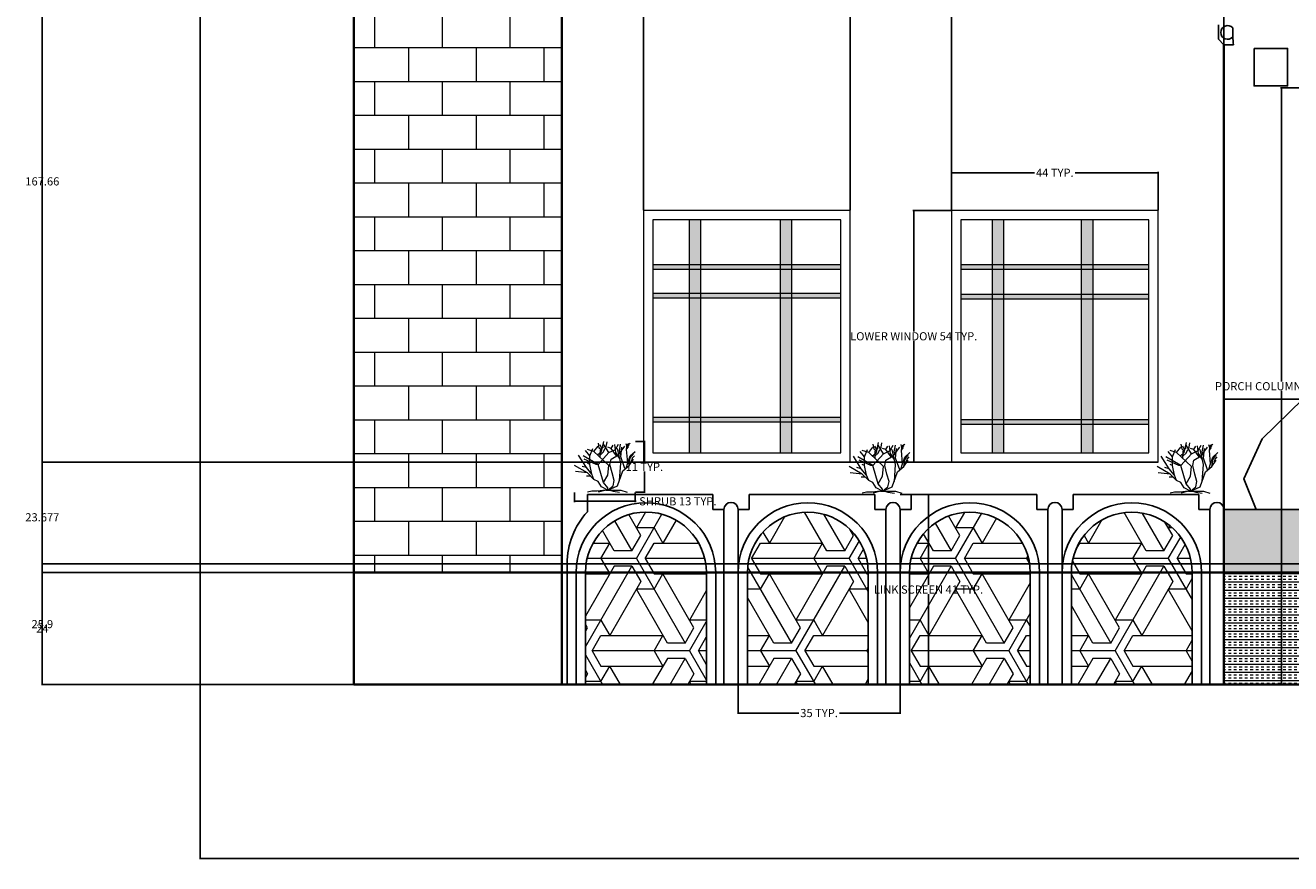
# Model space of a CAD drawing. Units: inches. Extents: x -17 to 741, y 7 to 490.
# Tile 1 of 8: x -17 to 254, y 14 to 193. Entities that reach past the tile are written whole.
import ezdxf

# ---------------------------------------------------------------- set-up
doc = ezdxf.new("R2010")
doc.units = ezdxf.units.IN
doc.header["$MEASUREMENT"] = 0
for name, color, linetype, lineweight in [('A-ANNO-DIMS', 2, 'Continuous', 18), ('A-ELEV-PATT', 252, 'Continuous', 13), ('A-FLOR-RAIL', 7, 'Continuous', 25), ('A-GLAZ', 4, 'Continuous', 18), ('A-ROOF-CNPE', 7, 'Continuous', 25), ('A-WALL', 7, 'Continuous', 35), ('A-WALL-PATT', 8, 'Continuous', 13), ('A-WALL-SCRN', 7, 'Continuous', 25), ('L-PLNT', 3, 'Continuous', 18)]:
    doc.layers.add(name, color=color, linetype=linetype, lineweight=lineweight)
doc.styles.get("Standard").update_dxf_attribs({"font": 'arial.ttf'})
doc.dimstyles.get("Standard").update_dxf_attribs({"dimtxt": 1.75, "dimasz": 0.18, "dimexe": 0.18, "dimexo": 0.0625, "dimgap": 0.09, "dimtad": 0, "dimtih": 1, "dimtoh": 1, "dimdec": 4, "dimzin": 0, "dimdsep": 46, "dimlunit": 4, "dimtxsty": 'Standard', "dimcen": 0.09, "dimadec": 0, "dimazin": 0, "dimtfac": 1, "dimtdec": 4, "dimtofl": 0, "dimtmove": 0, "dimatfit": 3, "dimfxl": 1, "dimtolj": 1, "dimtzin": 0, "dimarcsym": 0})

# ---------------------------------------------------------------- blocks, each defined once
blk = doc.blocks.new('Shrub - elevation')
for p, q in [((-11.433, 18.289), (-10.457, 22.749)), ((-16.8, 16.32), (-18.72, 18.72)), ((-14.88, 18.24), (-17.76, 19.2)), ((-16.8, 16.32), (-15.36, 19.68)), ((-14.88, 18.24), (-12.96, 20.64)), ((-8.16, 12), (-14.88, 18.24)), ((-13.325, 16.724), (-11.433, 18.289)), ((-12.96, 12.48), (-8.16, 17.76)), ((-12.471, 19.775), (-12.898, 22.044)), ((-11.677, 19.071), (-12.471, 19.775)), ((-11.28, 19.619), (-12.104, 21.184)), ((-12.043, 15.628), (-11.921, 18.836)), ((-11.982, 16.802), (-10.579, 18.054)), ((-11.921, 18.836), (-10.64, 20.401)), ((-10.579, 18.054), (-9.846, 19.697)), ((-8.16, 17.76), (-10.56, 21.6)), ((-9.48, 19.775), (-8.992, 22.592)), ((-7.2, 19.68), (-8.64, 20.16)), ((-8.16, 17.76), (-5.28, 19.2)), ((-7.2, 19.68), (-6.24, 21.12)), ((-4.8, 16.32), (-7.2, 19.68)), ((-5.086, 17.741), (-5.513, 21.34)), ((-5.28, 19.2), (-3.84, 21.6)), ((-3.377, 15.315), (-5.086, 17.819)), ((-2.88, 12.96), (-4.32, 19.68)), ((-3.84, 16.8), (-0.96, 20.64)), ((-3.377, 18.602), (-2.888, 21.575)), ((-2.766, 16.802), (-3.377, 18.602)), ((-2.88, 15.84), (-2.4, 20.16)), ((-0.508, 21.888), (-0.081, 20.558)), ((-0.203, 19.149), (0.102, 21.34)), ((0.346, 13.203), (-0.203, 19.149)), ((-0.142, 19.384), (0.59, 20.401)), ((-0.02, 20.01), (0.896, 21.105)), ((0.041, 20.714), (1.384, 22.044)), ((0.102, 21.34), (0.835, 21.888)), ((1.323, 16.254), (3.642, 18.289)), ((1.44, 15.36), (2.88, 17.28)), ((-17.76, 8.64), (-23.663, 11.961)), ((-18.24, 11.04), (-21.755, 16.655)), ((-18.24, 11.04), (-20.16, 11.52)), ((-12.96, 12.48), (-19.68, 16.32)), ((-13.92, 12.48), (-19.2, 14.88)), ((-16.8, 12.48), (-17.76, 12.96)), ((-16.8, 12.48), (-16.8, 16.32)), ((-15.84, 8.16), (-16.8, 12.48)), ((-12.96, 12.48), (-13.92, 12.48)), ((-10.56, 4.32), (-12.96, 12.48)), ((-8.64, 7.68), (-8.16, 12)), ((-7.68, 12.48), (-7.2, 14.88)), ((-6.72, 8.64), (-7.68, 12.48)), ((-7.2, 14.88), (-3.84, 16.8)), ((-3.36, 5.28), (-2.88, 12.96)), ((-0.96, 10.56), (-2.88, 15.84)), ((-1.92, 9.6), (0.96, 12)), ((-0.48, 10.8), (0.346, 13.203)), ((0.346, 13.203), (1.323, 16.254)), ((0.96, 12), (1.44, 15.36)), ((0.96, 12), (2.88, 14.88)), ((1.92, 13.44), (2.4, 15.36)), ((2.4, 15.36), (3.36, 16.32)), ((-17.76, 8.64), (-23.128, 9.222)), ((-15.84, 8.16), (-18.24, 11.04)), ((-16.32, 7.2), (-18.24, 7.2)), ((-14.88, 5.76), (-17.76, 8.64)), ((-14.88, 5.76), (-15.84, 8.16)), ((-12.96, 4.8), (-14.88, 5.76)), ((-10.56, 4.32), (-8.64, 7.68)), ((-5.76, 5.28), (-6.72, 8.64)), ((-4.32, 2.88), (-1.92, 9.6)), ((-15.84, 0.48), (-17.76, 0)), ((-13.44, 0.48), (-15.84, 0.48)), ((-9.6, 0.96), (-13.44, 0.48)), ((-11.52, 2.4), (-12.96, 4.8)), ((-9.6, 0.96), (-12.96, 0)), ((-8.64, 0.96), (-11.52, 2.4)), ((-8.64, 1.92), (-10.56, 4.32)), ((-9.6, 0.96), (-7.68, 0.96)), ((-8.64, 0.96), (-4.32, 2.88)), ((-8.64, 0.96), (-6.24, 2.88)), ((-8.64, 0.96), (-8.64, 1.92)), ((-8.64, 0.96), (-2.88, 0.96)), ((-7.68, 0.96), (-6.24, 0.48)), ((-6.24, 2.88), (-5.76, 5.28)), ((-6.24, 0.48), (-3.36, 0)), ((-2.88, 0.96), (0, 0))]:
    blk.add_line(p, q)
blk = doc.blocks.new('SCREEN-ARCH-END-BAY')
for p, q in [((4.33, 40.71), (4.33, 37.01)), ((4.33, 40.71), (31.23, 40.71)), ((31.23, 40.71), (31.23, 37.52)), ((31.23, 37.52), (33.14, 37.52)), ((33.14, 37.52), (33.61, 37.52)), ((33.61, 37.52), (33.61, 0)), ((36.63, 37.52), (36.63, 0)), ((0, 0), (0, 25.9))]:
    blk.add_line(p, q)
for points in [[(31.83, 0), (31.83, 24, 1), (1.92, 24), (1.92, 0)], [(29.83, 0), (29.83, 24, 1), (3.92, 24), (3.92, 0)]]:
    blk.add_lwpolyline(points, format="xyb")
for centre, radius, start in [((35.12, 37.52), 1.51, 0), ((16.41, 25.9), 16.41, 137.3839)]:
    blk.add_arc(centre, radius, start, 180)
blk = doc.blocks.new('SCREEN-ARCH-LINK-BAY')
for p, q in [((2.41, 40.71), (2.41, 37.52)), ((2.41, 40.71), (29.3, 40.71)), ((29.3, 40.71), (29.3, 37.52)), ((0, 37.52), (2.41, 37.52)), ((29.3, 37.52), (31.22, 37.52)), ((31.22, 37.52), (31.69, 37.52)), ((31.69, 37.52), (31.69, 0)), ((34.71, 37.52), (34.71, 0))]:
    blk.add_line(p, q)
for points in [[(29.9, 0), (29.9, 24, 1), (0, 24), (0, 0)], [(27.9, 0), (27.9, 24, 1), (2, 24), (2, 0)]]:
    blk.add_lwpolyline(points, format="xyb")
blk.add_arc((33.2, 37.52), 1.51, 0, 180)
blk = doc.blocks.new('WIN-ELEV-FRAME')
for points in [[(0, 0), (44.31, 0), (44.31, 53.92), (0, 53.92)], [(2, 2), (42.31, 2), (42.31, 51.92), (2, 51.92)]]:
    blk.add_lwpolyline(points, close=True)
blk = doc.blocks.new('PORCH-POINTED-PANEL')
for p, q in [((0, 23.66), (33.75, 23.66)), ((0, 0), (33.75, 0))]:
    blk.add_line(p, q)
blk.add_lwpolyline([(6.92, 0), (4.23, 6.56), (8.17, 15.14), (16.88, 23.66), (24.3, 16.07), (28.38, 7.1), (24.8, 0)])
blk = doc.blocks.new('*D21')
at = {"layer": 'A-ANNO-DIMS', "color": 0, "lineweight": -2, "transparency": 16777216}
for p, q in [((170.58, 92.72), (176.81, 92.72)), ((176.63, 92.54), (176.63, 73.36)), ((176.63, 52.19), (176.63, 71.37)), ((170.58, 52.01), (176.81, 52.01))]:
    blk.add_line(p, q, dxfattribs=at)
at = {"layer": 'A-ANNO-DIMS', "color": 0, "transparency": 16777216}
for points in [[(176.6, 92.54), (176.66, 92.54), (176.63, 92.72)], [(176.6, 52.19), (176.66, 52.19), (176.63, 52.01)]]:
    blk.add_solid(points, dxfattribs=at)
at = {"layer": 'Defpoints', "color": 0, "transparency": 16777216}
for p in [(170.52, 92.72), (176.63, 92.72), (170.52, 52.01)]:
    blk.add_point(p, dxfattribs=at)
at = {"layer": 'A-ANNO-DIMS', "color": 0, "transparency": 16777216, "insert": (176.63, 72.36), "char_height": 1.75, "attachment_point": 5}
blk.add_mtext('\\A1;LINK SCREEN 41 TYP.', dxfattribs=at)
blk = doc.blocks.new('*D22')
at = {"layer": 'A-ANNO-DIMS', "color": 0, "lineweight": -2, "transparency": 16777216}
for p, q in [((135.81, 51.95), (135.81, 45.72)), ((170.52, 51.95), (170.52, 45.72)), ((135.99, 45.9), (148.82, 45.9)), ((170.34, 45.9), (157.52, 45.9))]:
    blk.add_line(p, q, dxfattribs=at)
at = {"layer": 'A-ANNO-DIMS', "color": 0, "transparency": 16777216}
for points in [[(135.99, 45.93), (135.99, 45.87), (135.81, 45.9)], [(170.34, 45.93), (170.34, 45.87), (170.52, 45.9)]]:
    blk.add_solid(points, dxfattribs=at)
at = {"layer": 'Defpoints', "color": 0, "transparency": 16777216}
for p in [(135.81, 52.01), (170.52, 52.01), (170.52, 45.9)]:
    blk.add_point(p, dxfattribs=at)
at = {"layer": 'A-ANNO-DIMS', "color": 0, "transparency": 16777216, "insert": (153.17, 45.9), "char_height": 1.75, "attachment_point": 5}
blk.add_mtext('\\A1;35 TYP.', dxfattribs=at)
blk = doc.blocks.new('*D25')
at = {"layer": 'A-ANNO-DIMS', "color": 0, "lineweight": -2, "transparency": 16777216}
for p, q in [((181.48, 153.6), (173.27, 153.6)), ((173.45, 153.42), (173.45, 127.64)), ((173.45, 99.86), (173.45, 125.65)), ((181.48, 99.68), (173.27, 99.68))]:
    blk.add_line(p, q, dxfattribs=at)
at = {"layer": 'A-ANNO-DIMS', "color": 0, "transparency": 16777216}
for points in [[(173.42, 153.42), (173.48, 153.42), (173.45, 153.6)], [(173.42, 99.86), (173.48, 99.86), (173.45, 99.68)]]:
    blk.add_solid(points, dxfattribs=at)
at = {"layer": 'Defpoints', "color": 0, "transparency": 16777216}
for p in [(173.45, 153.6), (181.54, 153.6), (181.54, 99.68)]:
    blk.add_point(p, dxfattribs=at)
at = {"layer": 'A-ANNO-DIMS', "color": 0, "transparency": 16777216, "insert": (173.45, 126.64), "char_height": 1.75, "attachment_point": 5}
blk.add_mtext('\\A1;LOWER WINDOW 54 TYP.', dxfattribs=at)
blk = doc.blocks.new('*D26')
at = {"layer": 'A-ANNO-DIMS', "color": 0, "lineweight": -2, "transparency": 16777216}
for p, q in [((181.54, 153.67), (181.54, 161.87)), ((181.72, 161.69), (199.31, 161.69)), ((225.67, 161.69), (208.08, 161.69)), ((225.85, 153.67), (225.85, 161.87))]:
    blk.add_line(p, q, dxfattribs=at)
at = {"layer": 'A-ANNO-DIMS', "color": 0, "transparency": 16777216}
for points in [[(181.72, 161.72), (181.72, 161.66), (181.54, 161.69)], [(225.67, 161.72), (225.67, 161.66), (225.85, 161.69)]]:
    blk.add_solid(points, dxfattribs=at)
at = {"layer": 'Defpoints', "color": 0, "transparency": 16777216}
for p in [(225.85, 161.69), (181.54, 153.6), (225.85, 153.6)]:
    blk.add_point(p, dxfattribs=at)
at = {"layer": 'A-ANNO-DIMS', "color": 0, "transparency": 16777216, "insert": (203.69, 161.69), "char_height": 1.75, "attachment_point": 5}
blk.add_mtext('\\A1;44 TYP.', dxfattribs=at)
blk = doc.blocks.new('*D27')
at = {"layer": 'A-ANNO-DIMS', "color": 0, "lineweight": -2, "transparency": 16777216}
for p, q in [((271.37, 179.87), (252.08, 179.87)), ((252.26, 179.69), (252.26, 116.93)), ((252.26, 52.19), (252.26, 114.94)), ((271.37, 52.01), (252.08, 52.01))]:
    blk.add_line(p, q, dxfattribs=at)
at = {"layer": 'A-ANNO-DIMS', "color": 0, "transparency": 16777216}
for points in [[(252.23, 179.69), (252.29, 179.69), (252.26, 179.87)], [(252.23, 52.19), (252.29, 52.19), (252.26, 52.01)]]:
    blk.add_solid(points, dxfattribs=at)
at = {"layer": 'Defpoints', "color": 0, "transparency": 16777216}
for p in [(252.26, 179.87), (271.44, 179.87), (271.44, 52.01)]:
    blk.add_point(p, dxfattribs=at)
at = {"layer": 'A-ANNO-DIMS', "color": 0, "transparency": 16777216, "insert": (252.26, 115.94), "char_height": 1.75, "attachment_point": 5}
blk.add_mtext('\\A1;PORCH COLUMN 128 TYP.', dxfattribs=at)
blk = doc.blocks.new('*D33')
at = {"layer": 'A-ANNO-DIMS', "color": 0, "lineweight": -2, "transparency": 16777216}
for p, q in [((100.73, 93.17), (100.73, 91.1)), ((113.77, 93.17), (113.77, 91.1)), ((100.91, 91.28), (113.59, 91.28)), ((113.77, 91.28), (113.95, 91.28))]:
    blk.add_line(p, q, dxfattribs=at)
at = {"layer": 'A-ANNO-DIMS', "color": 0, "transparency": 16777216}
for points in [[(100.91, 91.31), (100.91, 91.25), (100.73, 91.28)], [(113.59, 91.31), (113.59, 91.25), (113.77, 91.28)]]:
    blk.add_solid(points, dxfattribs=at)
at = {"layer": 'Defpoints', "color": 0, "transparency": 16777216}
for p in [(100.73, 93.23), (113.77, 93.23), (113.77, 91.28)]:
    blk.add_point(p, dxfattribs=at)
at = {"layer": 'A-ANNO-DIMS', "color": 0, "transparency": 16777216, "insert": (122.91, 91.28), "char_height": 1.75, "attachment_point": 5}
blk.add_mtext('\\A1;SHRUB 13 TYP.', dxfattribs=at)
blk = doc.blocks.new('*D34')
at = {"layer": 'A-ANNO-DIMS', "color": 0, "lineweight": -2, "transparency": 16777216}
for p, q in [((113.83, 104.09), (115.91, 104.09)), ((115.73, 103.91), (115.73, 99.63)), ((115.73, 93.41), (115.73, 97.69)), ((113.83, 93.23), (115.91, 93.23))]:
    blk.add_line(p, q, dxfattribs=at)
at = {"layer": 'A-ANNO-DIMS', "color": 0, "transparency": 16777216}
for points in [[(115.7, 103.91), (115.76, 103.91), (115.73, 104.09)], [(115.7, 93.41), (115.76, 93.41), (115.73, 93.23)]]:
    blk.add_solid(points, dxfattribs=at)
at = {"layer": 'Defpoints', "color": 0, "transparency": 16777216}
for p in [(113.77, 104.09), (115.73, 104.09), (113.77, 93.23)]:
    blk.add_point(p, dxfattribs=at)
at = {"layer": 'A-ANNO-DIMS', "color": 0, "transparency": 16777216, "insert": (115.73, 98.66), "char_height": 1.75, "attachment_point": 5}
blk.add_mtext('\\A1;11 TYP.', dxfattribs=at)
blk = doc.blocks.new('*D37')
at = {"layer": 'A-ANNO-DIMS', "color": 0, "lineweight": -2, "transparency": 16777216}
for p, q in [((20.52, 396.95), (20.52, 14.58)), ((553.43, 51.95), (553.43, 14.58)), ((20.7, 14.76), (283.93, 14.76)), ((553.25, 14.76), (290.02, 14.76))]:
    blk.add_line(p, q, dxfattribs=at)
at = {"layer": 'A-ANNO-DIMS', "color": 0, "transparency": 16777216}
for points in [[(20.7, 14.79), (20.7, 14.73), (20.52, 14.76)], [(553.25, 14.79), (553.25, 14.73), (553.43, 14.76)]]:
    blk.add_solid(points, dxfattribs=at)
at = {"layer": 'Defpoints', "color": 0, "transparency": 16777216}
for p in [(20.52, 397.01), (553.43, 52.01), (553.43, 14.76)]:
    blk.add_point(p, dxfattribs=at)
at = {"layer": 'A-ANNO-DIMS', "color": 0, "transparency": 16777216, "insert": (286.97, 14.76), "char_height": 1.75, "attachment_point": 5}
blk.add_mtext('\\A1;532.9', dxfattribs=at)
blk = doc.blocks.new('*D39')
at = {"layer": 'A-ANNO-DIMS', "color": 0, "lineweight": -2, "transparency": 16777216}
for p, q in [((20.45, 410.82), (-13.46, 410.82)), ((-13.28, 410.64), (-13.28, 232.4)), ((-13.28, 52.19), (-13.28, 230.43)), ((53.4, 52.01), (-13.46, 52.01))]:
    blk.add_line(p, q, dxfattribs=at)
at = {"layer": 'A-ANNO-DIMS', "color": 0, "transparency": 16777216}
for points in [[(-13.31, 410.64), (-13.25, 410.64), (-13.28, 410.82)], [(-13.31, 52.19), (-13.25, 52.19), (-13.28, 52.01)]]:
    blk.add_solid(points, dxfattribs=at)
at = {"layer": 'Defpoints', "color": 0, "transparency": 16777216}
for p in [(-13.28, 410.82), (20.52, 410.82), (53.46, 52.01)]:
    blk.add_point(p, dxfattribs=at)
at = {"layer": 'A-ANNO-DIMS', "color": 0, "transparency": 16777216, "insert": (-13.28, 231.41), "char_height": 1.75, "attachment_point": 5}
blk.add_mtext('\\A1;358.8', dxfattribs=at)
blk = doc.blocks.new('*D48')
at = {"layer": 'A-ANNO-DIMS', "color": 0, "lineweight": -2, "transparency": 16777216}
for p, q in [((53.4, 76.01), (-13.46, 76.01)), ((-13.28, 75.83), (-13.28, 64.98)), ((-13.28, 52.19), (-13.28, 63.04)), ((53.4, 52.01), (-13.46, 52.01))]:
    blk.add_line(p, q, dxfattribs=at)
at = {"layer": 'A-ANNO-DIMS', "color": 0, "transparency": 16777216}
for points in [[(-13.31, 75.83), (-13.25, 75.83), (-13.28, 76.01)], [(-13.31, 52.19), (-13.25, 52.19), (-13.28, 52.01)]]:
    blk.add_solid(points, dxfattribs=at)
at = {"layer": 'Defpoints', "color": 0, "transparency": 16777216}
for p in [(-13.28, 76.01), (53.46, 76.01), (53.46, 52.01)]:
    blk.add_point(p, dxfattribs=at)
at = {"layer": 'A-ANNO-DIMS', "color": 0, "transparency": 16777216, "insert": (-13.28, 64.01), "char_height": 1.75, "attachment_point": 5}
blk.add_mtext('\\A1;24', dxfattribs=at)
blk = doc.blocks.new('*D49')
at = {"layer": 'A-ANNO-DIMS', "color": 0, "lineweight": -2, "transparency": 16777216}
for p, q in [((53.4, 243.67), (-13.46, 243.67)), ((-13.28, 243.49), (-13.28, 160.82)), ((-13.28, 76.19), (-13.28, 158.86)), ((53.4, 76.01), (-13.46, 76.01))]:
    blk.add_line(p, q, dxfattribs=at)
at = {"layer": 'A-ANNO-DIMS', "color": 0, "transparency": 16777216}
for points in [[(-13.31, 243.49), (-13.25, 243.49), (-13.28, 243.67)], [(-13.31, 76.19), (-13.25, 76.19), (-13.28, 76.01)]]:
    blk.add_solid(points, dxfattribs=at)
at = {"layer": 'Defpoints', "color": 0, "transparency": 16777216}
for p in [(-13.28, 243.67), (53.46, 243.67), (53.46, 76.01)]:
    blk.add_point(p, dxfattribs=at)
at = {"layer": 'A-ANNO-DIMS', "color": 0, "transparency": 16777216, "insert": (-13.28, 159.84), "char_height": 1.75, "attachment_point": 5}
blk.add_mtext('\\A1;167.66', dxfattribs=at)
blk = doc.blocks.new('*D51')
at = {"layer": 'A-ANNO-DIMS', "color": 0, "lineweight": -2, "transparency": 16777216}
for p, q in [((53.46, 52.07), (53.46, 488.55)), ((53.64, 488.37), (72.7, 488.37)), ((97.89, 488.37), (78.84, 488.37)), ((98.07, 52.07), (98.07, 488.55))]:
    blk.add_line(p, q, dxfattribs=at)
at = {"layer": 'A-ANNO-DIMS', "color": 0, "transparency": 16777216}
for points in [[(53.64, 488.4), (53.64, 488.34), (53.46, 488.37)], [(97.89, 488.4), (97.89, 488.34), (98.07, 488.37)]]:
    blk.add_solid(points, dxfattribs=at)
at = {"layer": 'Defpoints', "color": 0, "transparency": 16777216}
for p in [(98.07, 488.37), (53.46, 52.01), (98.07, 52.01)]:
    blk.add_point(p, dxfattribs=at)
at = {"layer": 'A-ANNO-DIMS', "color": 0, "transparency": 16777216, "insert": (75.77, 488.37), "char_height": 1.75, "attachment_point": 5}
blk.add_mtext('\\A1;44.62', dxfattribs=at)
blk = doc.blocks.new('*D52')
at = {"layer": 'A-ANNO-DIMS', "color": 0, "lineweight": -2, "transparency": 16777216}
for p, q in [((239.94, 113.25), (239.94, 488.55)), ((240.12, 488.37), (253.76, 488.37)), ((273.51, 488.37), (259.86, 488.37)), ((273.69, 113.25), (273.69, 488.55))]:
    blk.add_line(p, q, dxfattribs=at)
at = {"layer": 'A-ANNO-DIMS', "color": 0, "transparency": 16777216}
for points in [[(240.12, 488.4), (240.12, 488.34), (239.94, 488.37)], [(273.51, 488.4), (273.51, 488.34), (273.69, 488.37)]]:
    blk.add_solid(points, dxfattribs=at)
at = {"layer": 'Defpoints', "color": 0, "transparency": 16777216}
for p in [(273.69, 488.37), (239.94, 113.19), (273.69, 113.19)]:
    blk.add_point(p, dxfattribs=at)
at = {"layer": 'A-ANNO-DIMS', "color": 0, "transparency": 16777216, "insert": (256.81, 488.37), "char_height": 1.75, "attachment_point": 5}
blk.add_mtext('\\A1;33.75', dxfattribs=at)
blk = doc.blocks.new('*D58')
at = {"layer": 'A-ANNO-DIMS', "color": 0, "lineweight": -2, "transparency": 16777216}
for p, q in [((98.07, 52.07), (98.07, 488.55)), ((98.25, 488.37), (103.16, 488.37)), ((115.36, 488.37), (110.45, 488.37)), ((115.54, 153.67), (115.54, 488.55))]:
    blk.add_line(p, q, dxfattribs=at)
at = {"layer": 'A-ANNO-DIMS', "color": 0, "transparency": 16777216}
for points in [[(98.25, 488.4), (98.25, 488.34), (98.07, 488.37)], [(115.36, 488.4), (115.36, 488.34), (115.54, 488.37)]]:
    blk.add_solid(points, dxfattribs=at)
at = {"layer": 'Defpoints', "color": 0, "transparency": 16777216}
for p in [(115.54, 488.37), (115.54, 153.6), (98.07, 52.01)]:
    blk.add_point(p, dxfattribs=at)
at = {"layer": 'A-ANNO-DIMS', "color": 0, "transparency": 16777216, "insert": (106.81, 488.37), "char_height": 1.75, "attachment_point": 5}
blk.add_mtext('\\A1;17.465', dxfattribs=at)
blk = doc.blocks.new('*D59')
at = {"layer": 'A-ANNO-DIMS', "color": 0, "lineweight": -2, "transparency": 16777216}
for p, q in [((159.85, 153.67), (159.85, 488.55)), ((160.03, 488.37), (167.63, 488.37)), ((181.36, 488.37), (173.75, 488.37)), ((181.54, 153.67), (181.54, 488.55))]:
    blk.add_line(p, q, dxfattribs=at)
at = {"layer": 'A-ANNO-DIMS', "color": 0, "transparency": 16777216}
for points in [[(160.03, 488.4), (160.03, 488.34), (159.85, 488.37)], [(181.36, 488.4), (181.36, 488.34), (181.54, 488.37)]]:
    blk.add_solid(points, dxfattribs=at)
at = {"layer": 'Defpoints', "color": 0, "transparency": 16777216}
for p in [(181.54, 488.37), (159.85, 153.6), (181.54, 153.6)]:
    blk.add_point(p, dxfattribs=at)
at = {"layer": 'A-ANNO-DIMS', "color": 0, "transparency": 16777216, "insert": (170.69, 488.37), "char_height": 1.75, "attachment_point": 5}
blk.add_mtext('\\A1;21.69', dxfattribs=at)
blk = doc.blocks.new('*D61')
at = {"layer": 'A-ANNO-DIMS', "color": 0, "lineweight": -2, "transparency": 16777216}
for p, q in [((225.78, 99.68), (-13.46, 99.68)), ((-13.28, 99.5), (-13.28, 88.83)), ((-13.28, 76.19), (-13.28, 86.86)), ((299.72, 76.01), (-13.46, 76.01))]:
    blk.add_line(p, q, dxfattribs=at)
at = {"layer": 'A-ANNO-DIMS', "color": 0, "transparency": 16777216}
for points in [[(-13.31, 99.5), (-13.25, 99.5), (-13.28, 99.68)], [(-13.31, 76.19), (-13.25, 76.19), (-13.28, 76.01)]]:
    blk.add_solid(points, dxfattribs=at)
at = {"layer": 'Defpoints', "color": 0, "transparency": 16777216}
for p in [(225.85, 99.68), (-13.28, 76.01), (299.79, 76.01)]:
    blk.add_point(p, dxfattribs=at)
at = {"layer": 'A-ANNO-DIMS', "color": 0, "transparency": 16777216, "insert": (-13.28, 87.85), "char_height": 1.75, "attachment_point": 5}
blk.add_mtext('\\A1;23.677', dxfattribs=at)
blk = doc.blocks.new('*D64')
at = {"layer": 'A-ANNO-DIMS', "color": 0, "lineweight": -2, "transparency": 16777216}
for p, q in [((516.74, 77.91), (-13.46, 77.91)), ((-13.28, 77.73), (-13.28, 65.94)), ((-13.28, 52.19), (-13.28, 63.98)), ((516.74, 52.01), (-13.46, 52.01))]:
    blk.add_line(p, q, dxfattribs=at)
at = {"layer": 'A-ANNO-DIMS', "color": 0, "transparency": 16777216}
for points in [[(-13.31, 77.73), (-13.25, 77.73), (-13.28, 77.91)], [(-13.31, 52.19), (-13.25, 52.19), (-13.28, 52.01)]]:
    blk.add_solid(points, dxfattribs=at)
at = {"layer": 'Defpoints', "color": 0, "transparency": 16777216}
for p in [(-13.28, 77.91), (516.8, 77.91), (516.8, 52.01)]:
    blk.add_point(p, dxfattribs=at)
at = {"layer": 'A-ANNO-DIMS', "color": 0, "transparency": 16777216, "insert": (-13.28, 64.96), "char_height": 1.75, "attachment_point": 5}
blk.add_mtext('\\A1;25.9', dxfattribs=at)

msp = doc.modelspace()

# ---------------------------------------------------------------- hatches: boundary and pattern name
at = {"layer": 'A-ELEV-PATT'}
h = msp.add_hatch(color=256, dxfattribs=at)
h.dxf.hatch_style = 1
h.paths.add_polyline_path([(323.0665, 158.6389), (301.7867, 158.6389), (301.7867, 78.0082), (323.0665, 78.0082)])
h.paths.add_polyline_path([(318.3825, 145.2592), (318.3825, 85.0354), (307.7462, 85.0354), (307.7462, 145.2592)], flags=16)
h.paths.add_polyline_path([(344.3462, 158.6389), (323.0665, 158.6389), (323.0665, 78.0082), (344.3462, 78.0082)])
h.paths.add_polyline_path([(339.3004, 145.2592), (339.3004, 85.0354), (328.6642, 85.0354), (328.6642, 145.2592)], flags=16)
h.paths.add_polyline_path([(192.7233, 151.6028), (190.2672, 151.6028), (190.2672, 142.0361), (192.7233, 142.0361)])
h.paths.add_polyline_path([(192.7233, 141.0361), (190.2672, 141.0361), (190.2672, 135.6738), (192.7233, 135.6738)])
h.paths.add_polyline_path([(192.7233, 142.0361), (190.2672, 142.0361), (190.2672, 141.0361), (192.7233, 141.0361)])
h.paths.add_polyline_path([(209.3698, 142.0361), (192.7233, 142.0361), (192.7233, 141.0361), (209.3698, 141.0361)])
h.paths.add_polyline_path([(190.2672, 142.0361), (183.5379, 142.0361), (183.5379, 141.0361), (190.2672, 141.0361)])
h.paths.add_polyline_path([(190.2672, 135.6738), (183.5379, 135.6738), (183.5379, 134.6738), (190.2672, 134.6738)])
h.paths.add_polyline_path([(192.7233, 135.6738), (190.2672, 135.6738), (190.2672, 134.6738), (192.7233, 134.6738)])
h.paths.add_polyline_path([(192.7233, 134.6738), (190.2672, 134.6738), (190.2672, 101.6848), (192.7233, 101.6848)])
h.paths.add_polyline_path([(209.3698, 135.6738), (192.7233, 135.6738), (192.7233, 134.6738), (209.3698, 134.6738)])
h.paths.add_polyline_path([(211.8259, 135.6738), (209.3698, 135.6738), (209.3698, 134.6738), (211.8259, 134.6738)])
h.paths.add_polyline_path([(211.8259, 141.0361), (209.3698, 141.0361), (209.3698, 135.6738), (211.8259, 135.6738)])
h.paths.add_polyline_path([(211.8259, 142.0361), (209.3698, 142.0361), (209.3698, 141.0361), (211.8259, 141.0361)])
h.paths.add_polyline_path([(211.8259, 151.6028), (209.3698, 151.6028), (209.3698, 142.0361), (211.8259, 142.0361)])
h.paths.add_polyline_path([(223.8474, 142.0361), (211.8259, 142.0361), (211.8259, 141.0361), (223.8474, 141.0361)])
h.paths.add_polyline_path([(223.8474, 135.6738), (211.8259, 135.6738), (211.8259, 134.6738), (223.8474, 134.6738)])
h.paths.add_polyline_path([(211.8259, 134.6738), (209.3698, 134.6738), (209.3698, 108.8153), (211.8259, 108.8153)])
h.paths.add_polyline_path([(211.8259, 108.8153), (209.3698, 108.8153), (209.3698, 107.8153), (211.8259, 107.8153)])
h.paths.add_polyline_path([(211.8259, 107.8153), (209.3698, 107.8153), (209.3698, 101.6848), (211.8259, 101.6848)])
h.paths.add_polyline_path([(223.8474, 108.8153), (211.8259, 108.8153), (211.8259, 107.8153), (223.8474, 107.8153)])
h.paths.add_polyline_path([(209.3698, 108.8153), (192.7233, 108.8153), (192.7233, 107.8153), (209.3698, 107.8153)])
h.paths.add_polyline_path([(190.2672, 108.8153), (183.5379, 108.8153), (183.5379, 107.8153), (190.2672, 107.8153)])
h.paths.add_polyline_path([(147.2864, 151.6028), (144.8304, 151.6028), (144.8304, 109.315), (147.2864, 109.315)])
h.paths.add_polyline_path([(147.2864, 109.315), (144.8304, 109.315), (144.8304, 108.315), (147.2864, 108.315)])
h.paths.add_polyline_path([(147.2864, 108.315), (144.8304, 108.315), (144.8304, 101.6848), (147.2864, 101.6848)])
h.paths.add_polyline_path([(157.8499, 109.315), (147.2864, 109.315), (147.2864, 108.315), (157.8499, 108.315)])
h.paths.add_polyline_path([(144.8304, 109.315), (127.7745, 109.315), (127.7745, 108.315), (144.8304, 108.315)])
h.paths.add_polyline_path([(127.7745, 109.315), (125.3184, 109.315), (125.3184, 108.315), (127.7745, 108.315)])
h.paths.add_polyline_path([(127.7745, 151.6028), (125.3184, 151.6028), (125.3184, 109.315), (127.7745, 109.315)])
h.paths.add_polyline_path([(125.3184, 109.315), (117.5405, 109.315), (117.5405, 108.315), (125.3184, 108.315)])
h.paths.add_polyline_path([(127.7745, 108.315), (125.3184, 108.315), (125.3184, 101.6848), (127.7745, 101.6848)])
h.paths.add_polyline_path([(125.3184, 135.9009), (117.5405, 135.9009), (117.5405, 134.9009), (125.3184, 134.9009)])
h.paths.add_polyline_path([(144.8304, 135.9009), (127.7745, 135.9009), (127.7745, 134.9009), (144.8304, 134.9009)])
h.paths.add_polyline_path([(157.8499, 135.9009), (147.2864, 135.9009), (147.2864, 134.9009), (157.8499, 134.9009)])
h.paths.add_polyline_path([(144.8304, 142.0361), (127.7745, 142.0361), (127.7745, 141.0361), (144.8304, 141.0361)])
h.paths.add_polyline_path([(157.8499, 142.0361), (147.2864, 142.0361), (147.2864, 141.0361), (157.8499, 141.0361)])
h.paths.add_polyline_path([(125.3184, 142.0361), (117.5405, 142.0361), (117.5405, 141.0361), (125.3184, 141.0361)])
h.paths.add_polyline_path([(447.5234, 311.9659), (445.0673, 311.9659), (445.0673, 302.3991), (447.5234, 302.3991)])
h.paths.add_polyline_path([(447.5234, 302.3991), (445.0673, 302.3991), (445.0673, 301.3991), (447.5234, 301.3991)])
h.paths.add_polyline_path([(458.0869, 302.3991), (447.5234, 302.3991), (447.5234, 301.3991), (458.0869, 301.3991)])
h.paths.add_polyline_path([(447.5234, 301.3991), (445.0673, 301.3991), (445.0673, 296.2639), (447.5234, 296.2639)])
h.paths.add_polyline_path([(447.5234, 296.2639), (445.0673, 296.2639), (445.0673, 295.2639), (447.5234, 295.2639)])
h.paths.add_polyline_path([(458.0869, 296.2639), (447.5234, 296.2639), (447.5234, 295.2639), (458.0869, 295.2639)])
h.paths.add_polyline_path([(445.0673, 296.2639), (428.0115, 296.2639), (428.0115, 295.2639), (445.0673, 295.2639)])
h.paths.add_polyline_path([(447.5234, 295.2639), (445.0673, 295.2639), (445.0673, 262.0479), (447.5234, 262.0479)])
h.paths.add_polyline_path([(445.0673, 302.3991), (428.0115, 302.3991), (428.0115, 301.3991), (445.0673, 301.3991)])
h.paths.add_polyline_path([(428.0115, 302.3991), (425.5554, 302.3991), (425.5554, 301.3991), (428.0115, 301.3991)])
h.paths.add_polyline_path([(428.0115, 311.9659), (425.5554, 311.9659), (425.5554, 302.3991), (428.0115, 302.3991)])
h.paths.add_polyline_path([(425.5554, 302.3991), (417.7774, 302.3991), (417.7774, 301.3991), (425.5554, 301.3991)])
h.paths.add_polyline_path([(428.0115, 301.3991), (425.5554, 301.3991), (425.5554, 296.2639), (428.0115, 296.2639)])
h.paths.add_polyline_path([(425.5554, 296.2639), (417.7774, 296.2639), (417.7774, 295.2639), (425.5554, 295.2639)])
h.paths.add_polyline_path([(428.0115, 296.2639), (425.5554, 296.2639), (425.5554, 295.2639), (428.0115, 295.2639)])
h.paths.add_polyline_path([(428.0115, 295.2639), (425.5554, 295.2639), (425.5554, 262.0479), (428.0115, 262.0479)])
h.paths.add_polyline_path([(425.5554, 269.8939), (417.7774, 269.8939), (417.7774, 268.8939), (425.5554, 268.8939)])
h.paths.add_polyline_path([(445.0673, 269.8939), (428.0115, 269.8939), (428.0115, 268.8939), (445.0673, 268.8939)])
h.paths.add_polyline_path([(458.0869, 269.8939), (447.5234, 269.8939), (447.5234, 268.8939), (458.0869, 268.8939)])
at = {"layer": 'A-WALL-PATT'}
h = msp.add_hatch(dxfattribs=at)
h.set_pattern_fill('BRICK', color=256, scale=29)
h.paths.add_polyline_path([(98.075, 232.0082), (98.075, 243.669), (86.0039, 243.669), (82.1639, 243.189), (79.7639, 243.189), (77.6592, 242.6628), (74.6406, 243.669), (68.8806, 243.669), (67.9206, 243.669), (53.4591, 243.669), (53.4591, 220.0082), (53.4591, 76.0082), (98.075, 76.0082)])
h = msp.add_hatch(dxfattribs=at)
h.set_pattern_fill('EARTH', color=256, scale=13, angle=16)
h.paths.add_polyline_path([(273.6893, 89.5255), (239.9367, 89.5255), (239.9367, 76.0082), (273.6893, 76.0082)])
h.paths.add_polyline_path([(394.976, 89.5255), (361.2234, 89.5255), (361.2234, 76.0082), (394.976, 76.0082)])
h.paths.add_polyline_path([(428.7285, 89.5255), (394.976, 89.5255), (394.976, 76.0082), (428.7285, 76.0082)])
h.paths.add_polyline_path([(460.302, 89.5255), (428.7285, 89.5255), (428.7285, 76.0082), (460.302, 76.0082)])
h.paths.add_polyline_path([(239.9367, 220.0082), (98.075, 220.0082), (98.075, 212.3604), (237.0146, 212.3604)])
h = msp.add_hatch(dxfattribs=at)
h.set_pattern_fill('ESCHER', color=256, scale=19)
h.paths.add_polyline_path([(129.0102, 76.0082), (103.1073, 76.0082), (103.1073, 52.0082), (129.0102, 52.0082)])
h.paths.add_polyline_path([(103.1073, 76.0082), (129.0102, 76.0082, 1)])
h.paths.add_polyline_path([(137.8147, 76.0082), (163.7176, 76.0082, 1)])
h.paths.add_polyline_path([(163.7176, 76.0082), (137.8147, 76.0082), (137.8147, 52.0082), (163.7176, 52.0082)])
h.paths.add_polyline_path([(172.522, 76.0082), (198.425, 76.0082, 1)])
h.paths.add_polyline_path([(198.425, 76.0082), (172.522, 76.0082), (172.522, 52.0082), (198.425, 52.0082)])
h.paths.add_polyline_path([(207.2294, 76.0082), (233.1323, 76.0082, 1)])
h.paths.add_polyline_path([(233.1323, 76.0082), (207.2294, 76.0082), (207.2294, 52.0082), (233.1323, 52.0082)])
h = msp.add_hatch(dxfattribs=at)
h.set_pattern_fill('INSUL', color=256, scale=4.7)
h.paths.add_polyline_path([(273.6893, 76.0082), (239.9367, 76.0082), (239.9367, 52.0082), (273.6893, 52.0082)])

# ---------------------------------------------------------------- linework, layer by layer
at = {"layer": 'A-GLAZ'}
for p, q in [((125.3184, 151.6028), (125.3184, 101.6848)), ((127.7745, 151.6028), (127.7745, 101.6848)), ((144.8304, 151.6028), (144.8304, 101.6848)), ((147.2864, 151.6028), (147.2864, 101.6848)), ((190.2672, 151.6028), (190.2672, 101.6848)), ((192.7233, 151.6028), (192.7233, 101.6848)), ((209.3698, 151.6028), (209.3698, 101.6848)), ((211.8259, 151.6028), (211.8259, 101.6848)), ((117.5405, 142.0361), (157.8499, 142.0361)), ((117.5405, 141.0361), (157.8499, 141.0361)), ((183.5379, 142.0361), (223.8474, 142.0361)), ((183.5379, 141.0361), (223.8474, 141.0361)), ((117.5405, 135.9009), (157.8499, 135.9009)), ((183.5379, 135.6738), (223.8474, 135.6738)), ((117.5405, 134.9009), (157.8499, 134.9009)), ((183.5379, 134.6738), (223.8474, 134.6738)), ((117.5405, 109.315), (157.8499, 109.315)), ((183.5379, 108.8153), (223.8474, 108.8153)), ((117.5405, 108.315), (157.8499, 108.315)), ((183.5379, 107.8153), (223.8474, 107.8153))]:
    msp.add_line(p, q, dxfattribs=at)
at = {"layer": 'A-ROOF-CNPE'}
for p, q in [((238.7685, 190.3139), (238.7685, 193.3539)), ((241.8149, 190.8921), (241.8149, 192.7208)), ((239.9367, 189.1301), (238.7685, 190.3139)), ((241.8996, 189.5254), (241.8149, 190.8921)), ((239.9367, 189.1301), (242.0022, 189.1301)), ((242.0022, 189.1301), (241.8996, 189.5254))]:
    msp.add_line(p, q, dxfattribs=at)
msp.add_lwpolyline([(246.3845, 188.3373), (253.5789, 188.3373), (253.5789, 180.2979), (246.3845, 180.2979)], close=True, dxfattribs=at)
msp.add_arc((240.7126, 191.758), 1.4636, 41.137671, 319.197435, dxfattribs=at)
at = {"layer": 'A-WALL'}
for p, q in [((98.075, 52.0082), (98.075, 232.0082)), ((53.4591, 76.0082), (53.4591, 220.0082)), ((239.9367, 52.0082), (239.9367, 189.1301)), ((53.4591, 76.0082), (361.2234, 76.0082)), ((53.4591, 76.0082), (53.4591, 52.0082)), ((53.4591, 52.0082), (280.0481, 52.0082))]:
    msp.add_line(p, q, dxfattribs=at)

# ---------------------------------------------------------------- block references
at = {"layer": 'A-FLOR-RAIL'}
msp.add_blockref('PORCH-POINTED-PANEL', (239.937, 89.526), dxfattribs=at)
at = {"layer": 'A-GLAZ'}
for p in [(115.54, 99.685), (181.5375, 99.685)]:
    msp.add_blockref('WIN-ELEV-FRAME', p, dxfattribs=at)
at = {"layer": 'A-WALL-SCRN'}
for name, p in [('SCREEN-ARCH-END-BAY', (99.184, 52.008)), ('SCREEN-ARCH-LINK-BAY', (135.815, 52.008)), ('SCREEN-ARCH-LINK-BAY', (170.5224, 52.008)), ('SCREEN-ARCH-LINK-BAY', (205.2297, 52.008))]:
    msp.add_blockref(name, p, dxfattribs=at)
at = {"layer": 'L-PLNT', "xscale": 0.4774719091281041, "yscale": 0.4774719091281041, "zscale": 0.4774719091281041}
for p in [(112.0324, 93.2309), (170.908, 92.9927), (236.8996, 92.9927)]:
    msp.add_blockref('Shrub - elevation', p, dxfattribs=at)

# ---------------------------------------------------------------- dimensions: what is measured, and where the dimension line sits
at = {"layer": 'A-ANNO-DIMS'}
for base, p1, p2, override, picture, middle in [((98.075, 488.3717), (53.4591, 52.0082), (98.075, 52.0082), {"dimdec": 2, "dimlfac": 1, "dimrnd": 0, "dimzin": 0, "dimdsep": 46, "dimlunit": 2}, '*D51', (75.7671, 488.3717)), ((115.54046, 488.37169), (98.07499, 52.00816), (115.54046, 153.60279), {"dimdec": 3, "dimlfac": 1, "dimrnd": 0, "dimzin": 0, "dimdsep": 46, "dimlunit": 2}, '*D58', (106.80773, 488.37169)), ((181.5379, 488.3717), (159.8499, 153.6028), (181.5379, 153.6028), {"dimdec": 2, "dimlfac": 1, "dimrnd": 0, "dimzin": 0, "dimdsep": 46, "dimlunit": 2}, '*D59', (170.6939, 488.3717)), ((273.6893, 488.3717), (239.9367, 113.1863), (273.6893, 113.1863), {"dimdec": 2, "dimlfac": 1, "dimrnd": 0, "dimzin": 0, "dimdsep": 46, "dimlunit": 2}, '*D52', (256.813, 488.3717)), ((553.4286, 14.7597), (20.5169, 397.0087), (553.4286, 52.0082), {"dimdec": 1, "dimlfac": 1, "dimrnd": 0, "dimzin": 0, "dimdsep": 46, "dimlunit": 2}, '*D37', (286.9727, 14.7597))]:
    dim = msp.add_linear_dim(base=base, p1=p1, p2=p2, dimstyle='Standard', override=override, dxfattribs=at)
    dim.commit()
    dim.dimension.update_dxf_attribs({"geometry": picture, "text_midpoint": middle})
for base, p1, p2, override, picture, middle in [((-13.2831, 410.8173), (53.4591, 52.0082), (20.5169, 410.8173), {"dimdec": 1, "dimlfac": 1, "dimrnd": 0, "dimzin": 0, "dimdsep": 46, "dimlunit": 2}, '*D39', (-13.2831, 231.4127)), ((-13.2831, 243.669), (53.4591, 76.0082), (53.4591, 243.669), {"dimdec": 2, "dimlfac": 1, "dimrnd": 0, "dimzin": 0, "dimdsep": 46, "dimlunit": 2}, '*D49', (-13.2831, 159.8386)), ((-13.2831, 76.0082), (225.8474, 99.6848), (299.7867, 76.0082), {"dimdec": 3, "dimlfac": 1, "dimrnd": 0, "dimzin": 0, "dimdsep": 46, "dimlunit": 2}, '*D61', (-13.2831, 87.8465)), ((-13.2831, 77.9092), (516.7979, 52.0082), (516.7979, 77.9092), {"dimdec": 1, "dimlfac": 1, "dimrnd": 0, "dimzin": 0, "dimdsep": 46, "dimlunit": 2}, '*D64', (-13.2831, 64.9587)), ((-13.2831, 76.0082), (53.4591, 52.0082), (53.4591, 76.0082), {"dimdec": 0, "dimlfac": 1, "dimrnd": 0, "dimzin": 0, "dimdsep": 46, "dimlunit": 2}, '*D48', (-13.2831, 64.0082))]:
    dim = msp.add_linear_dim(base=base, p1=p1, p2=p2, angle=90, dimstyle='Standard', override=override, dxfattribs=at)
    dim.commit()
    dim.dimension.update_dxf_attribs({"geometry": picture, "text_midpoint": middle})
for base, p1, p2, text, picture, middle in [((252.2574, 179.8702), (271.4367, 52.0082), (271.4367, 179.8702), 'PORCH COLUMN <> TYP.', '*D27', (252.2574, 115.9392)), ((173.4502, 153.6028), (181.5379, 99.6848), (181.5379, 153.6028), 'LOWER WINDOW <> TYP.', '*D25', (173.4502, 126.6438)), ((115.7269, 104.0929), (113.7713, 93.2309), (113.7713, 104.0929), '<> TYP.', '*D34', (115.7269, 98.6619)), ((176.6284, 92.7171), (170.522, 52.0082), (170.522, 92.7171), 'LINK SCREEN <> TYP.', '*D21', (176.6284, 72.3627))]:
    dim = msp.add_linear_dim(base=base, p1=p1, p2=p2, angle=90, text=text, dimstyle='Standard', override={"dimdec": 0, "dimlfac": 1, "dimrnd": 0, "dimzin": 0, "dimdsep": 46, "dimlunit": 2}, dxfattribs=at)
    dim.commit()
    dim.dimension.update_dxf_attribs({"geometry": picture, "text_midpoint": middle})
for base, p1, p2, text, picture, middle in [((225.8474, 161.6905), (181.5379, 153.6028), (225.8474, 153.6028), '<> TYP.', '*D26', (203.6927, 161.6905)), ((113.7713, 91.2753), (100.7339, 93.2309), (113.7713, 93.2309), 'SHRUB <> TYP.', '*D33', (122.9149, 91.2753)), ((170.522, 45.9018), (135.8147, 52.0082), (170.522, 52.0082), '<> TYP.', '*D22', (153.1684, 45.9018))]:
    dim = msp.add_linear_dim(base=base, p1=p1, p2=p2, text=text, dimstyle='Standard', override={"dimdec": 0, "dimlfac": 1, "dimrnd": 0, "dimzin": 0, "dimdsep": 46, "dimlunit": 2}, dxfattribs=at)
    dim.commit()
    dim.dimension.update_dxf_attribs({"geometry": picture, "text_midpoint": middle})

doc.saveas('drawing.dxf')
